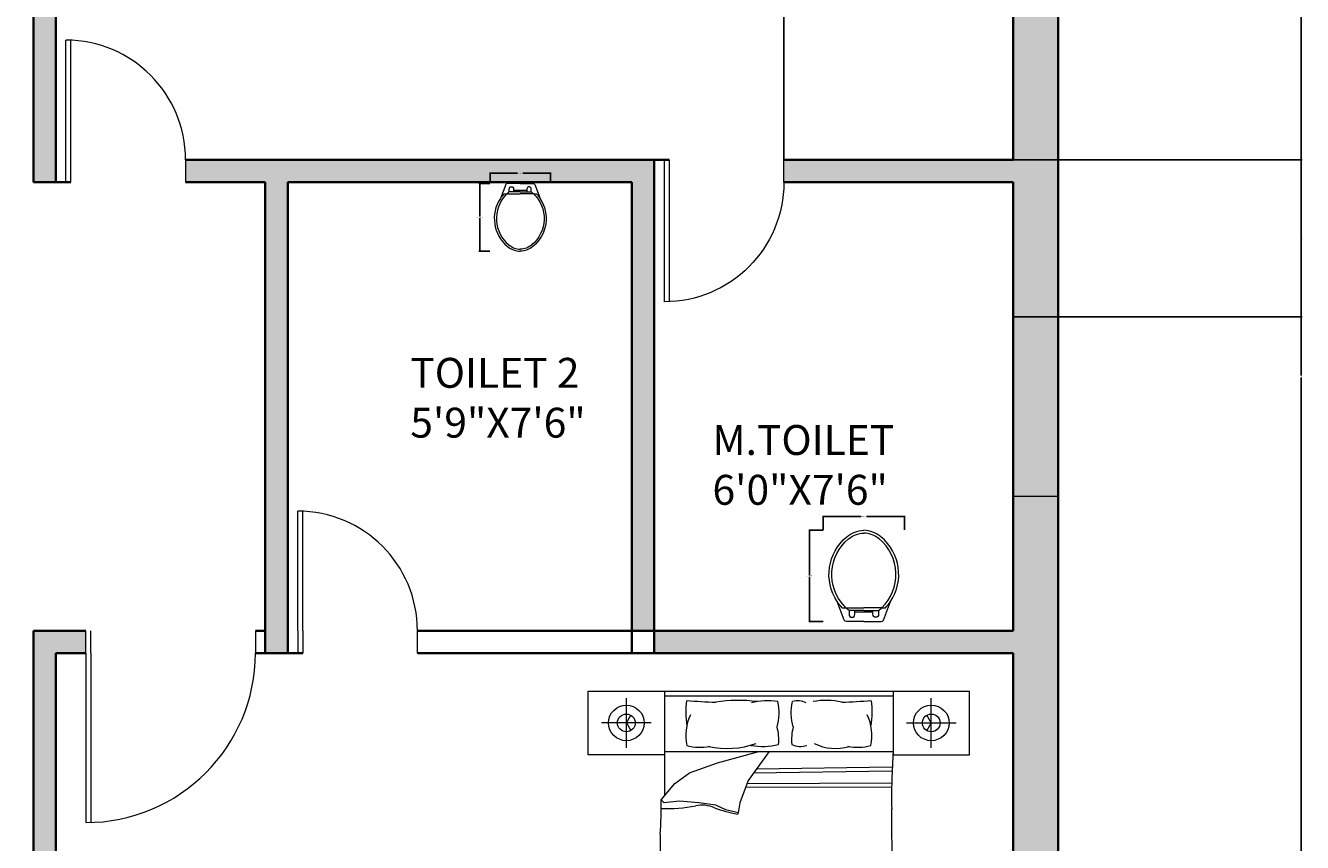
# Model space of a CAD drawing. Units: inches. Extents: x -26 to 13070, y -956 to 6917.
# Tile 4 of 13: x 341 to 597, y -760 to -596. Entities that reach past the tile are written whole.
import ezdxf

# ---------------------------------------------------------------- set-up
doc = ezdxf.new("R2010")
doc.units = ezdxf.units.IN
doc.header["$MEASUREMENT"] = 0
for name, color, linetype, lineweight in [('A-ANNO-DIMS', 2, 'Continuous', 18), ('A-AREA-IDEN', 7, 'Continuous', 18), ('A-DOOR', 3, 'Continuous', 18), ('A-FLOR-FIXT', 9, 'Continuous', 18), ('A-FURN', 8, 'Continuous', 13), ('A-GLAZ', 4, 'Continuous', 18), ('A-GLAZ-PATT', 8, 'Continuous', 13), ('A-WALL', 7, 'Continuous', 35), ('A-WALL-PATT', 252, 'Continuous', 13)]:
    doc.layers.add(name, color=color, linetype=linetype, lineweight=lineweight)
doc.styles.get("Standard").update_dxf_attribs({"font": 'arial.ttf'})
doc.dimstyles.get("Standard").update_dxf_attribs({"dimtxt": 0.18, "dimasz": 0.18, "dimexe": 0.18, "dimexo": 0.0625, "dimgap": 0.09, "dimtad": 0, "dimtih": 1, "dimtoh": 1, "dimdec": 0, "dimzin": 0, "dimdsep": 46, "dimlunit": 3, "dimtxsty": 'Standard', "dimcen": 0.09, "dimadec": 0, "dimazin": 0, "dimtfac": 1, "dimtdec": 0, "dimtofl": 0, "dimtmove": 0, "dimatfit": 3, "dimfxl": 1, "dimtolj": 1, "dimtzin": 0, "dimarcsym": 0})

# ---------------------------------------------------------------- blocks, each defined once
blk = doc.blocks.new('BED-DOUBLE-NIGHTSTANDS')
for p, q in [((0, 65), (76.43, 65)), ((15.29, 65), (15.29, 44.02)), ((7.64, 53.64), (7.64, 63.62)), ((61.14, 64.02), (15.29, 64.02)), ((68.79, 53.64), (68.79, 63.62)), ((12.64, 58.63), (2.65, 58.63)), ((63.79, 58.63), (73.78, 58.63)), ((15.29, 52.92), (61.14, 52.92)), ((25.9, 50.65), (34.24, 52.92)), ((36.28, 52.92), (32.09, 47.09)), ((20.33, 48.64), (25.9, 50.65)), ((60.91, 48.96), (33.16, 48.57)), ((60.94, 49.74), (33.73, 49.36)), ((14.6, 43.22), (17.39, 46.47)), ((17.39, 46.47), (20.33, 48.64)), ((32.09, 47.09), (30.39, 42.6)), ((60.87, 46.55), (31.85, 46.44)), ((60.87, 45.77), (31.55, 45.65)), ((15.22, 42.6), (14.6, 43.22)), ((18.32, 42.91), (15.22, 42.6)), ((22.19, 42.6), (18.32, 42.91)), ((25.59, 42.14), (22.19, 42.6)), ((27.6, 41.21), (25.59, 42.14)), ((30.08, 40.59), (27.6, 41.21)), ((30.39, 42.6), (30.08, 40.59)), ((10.09, 27.53), (14.41, 27.53)), ((10.09, 0), (10.09, 27.53)), ((14.41, 26.65), (10.97, 26.65)), ((10.97, 26.65), (10.97, 0.89)), ((64.92, 26.65), (61.55, 26.65)), ((61.57, 27.53), (65.81, 27.53)), ((64.92, 0.89), (64.92, 26.65)), ((65.81, 27.53), (65.81, 0)), ((61.56, 21.81), (14.4, 21.81)), ((61.49, 22.77), (14.41, 22.77)), ((53.73, 14.3), (22.7, 14.3)), ((18.51, 8.63), (18.34, 9.5)), ((23.85, 8.63), (24.02, 9.5)), ((52.05, 8.63), (51.88, 9.5)), ((57.39, 8.63), (57.56, 9.5)), ((10.97, 0.89), (64.92, 0.89)), ((65.81, 0), (10.09, 0))]:
    blk.add_line(p, q)
for points in [[(15.29, 52.26), (0, 52.26), (0, 65)], [(61.14, 65), (61.14, 52.26), (76.43, 52.26), (76.43, 65)], [(7.64, 58.63), (8.53, 60.17)], [(68.79, 58.63), (67.89, 60.17)], [(7.64, 58.63), (8.53, 57.08)], [(68.79, 58.63), (67.89, 57.08)]]:
    blk.add_lwpolyline(points)
for points in [[(19.68, 63.09, 0.074897), (19.77, 58.1, -0.472817)], [(37.86, 57.82, 0.14099), (38.01, 62.91, 0.235245)], [(41.12, 57.82, -0.14099), (40.97, 62.91, -0.235245)], [(56.75, 63.09, -0.074897), (56.66, 58.1, 0.472817)], [(14.44, 36.22, 0.001242), (14.4, 21.72, -0.127202), (12.87, 14.5)], [(61.47, 23.37, 0.056112), (62.02, 19.16, 0.095341), (63.1, 15.11)]]:
    blk.add_lwpolyline(points, format="xyb")
for centre, radius in [((7.64, 58.63), 3.57), ((68.79, 58.63), 3.57), ((7.64, 58.63), 1.78), ((68.79, 58.63), 1.78), ((22.92, 5.86), 0.195), ((52.98, 5.86), 0.195), ((21.65, 3.81), 0.195), ((54.25, 3.81), 0.195)]:
    blk.add_circle(centre, radius)
for centre, radius, start, end in [((61.8, 790.45), 728.57, 266.68521, 267.14978), ((30.15, 35.44), 27.72, 82.2196, 99.497), ((36, 49.44), 13.62, 81.5249, 103.96), ((42.02, 59.28), 3.78, 63.3437, 106.1026), ((47.68, 49.72), 13.44, 76.3427, 101.1841), ((14.63, 790.45), 728.57, 272.85022, 273.31479), ((29.41, 56.1), 9.85, 155.1316, 191.7583), ((47.02, 56.1), 9.85, 348.2417, 24.8684), ((28.85, 55.27), 9.36, 354.0129, 15.8293), ((50.13, 55.27), 9.36, 164.1707, 185.9871), ((22.4, 63.99), 10.24, 255.1039, 281.0369), ((27.79, 71.27), 17.76, 258.0397, 289.2615), ((34.99, 67.39), 13.48, 259.8617, 283.6238), ((42.53, 57.96), 4.05, 245.0183, 288.5407), ((49.61, 63.23), 9.73, 243.8761, 286.1746), ((54.03, 63.99), 10.24, 258.9631, 284.8961), ((198.16, 43.58), 137.33, 176.1, 180.9282), ((-55.48, 41.32), 70.1, 355.8294, 1.553), ((15.91, 70.29), 28.85, 267.4519, 281.3392), ((22.8, 35.91), 6.22, 66.2616, 101.3392), ((35.39, 69.47), 29.64, 250.1194, 259.3383), ((239.96, 38.59), 179.14, 179.1145, 184.8735), ((29.91, 40.53), 0.184, 268.8623, 19.7536), ((13.58, 14.54), 0.705, 183.98, 297.3412), ((21.79, -65.25), 79.56, 89.3433, 95.6887), ((16.65, 11.7), 1.29, 84.4856, 181.0538), ((13.28, 8.92), 5.78, 33.6671, 63.2997), ((16.25, 10.75), 2.3, 355.2933, 76.921), ((21.03, 12.36), 2.95, 145.785, 184.7304), ((15.4, 13.74), 3.17, 328.8218, 9.1554), ((19.32, 13.46), 0.92, 120.0293, 142.325), ((17.85, 12.92), 2.44, 289.2822, 29.1751), ((17.48, 12.48), 2.2, 7.436, 29.9149), ((18.93, 13.64), 1.14, 311.5653, 23.8354), ((19.32, 13.46), 0.92, 44.4517, 63.558), ((24.5, 12.92), 2.44, 150.8249, 250.7178), ((23.42, 13.64), 1.14, 156.1646, 228.4347), ((23.03, 13.46), 0.92, 113.229, 135.5483), ((24.87, 12.48), 2.2, 150.0851, 172.564), ((23.03, 13.46), 0.92, 37.675, 66.7144), ((21.32, 12.36), 2.95, 355.2696, 34.215), ((26.95, 13.74), 3.17, 169.7133, 211.1782), ((26.1, 10.75), 2.3, 103.079, 184.7067), ((29.07, 8.92), 5.78, 111.4941, 146.3329), ((25.7, 11.7), 1.29, 358.9462, 95.5144), ((50.19, 11.7), 1.29, 84.4856, 181.0538), ((46.82, 8.92), 5.78, 33.6671, 68.5059), ((49.8, 10.75), 2.3, 355.2933, 76.921), ((54.57, 12.36), 2.95, 145.785, 184.7304), ((48.94, 13.74), 3.17, 328.8218, 10.2867), ((52.87, 13.46), 0.92, 113.2856, 142.325), ((51.4, 12.92), 2.44, 289.2822, 29.1751), ((51.03, 12.48), 2.2, 7.436, 29.9149), ((52.87, 13.46), 0.92, 44.4517, 66.7144), ((52.48, 13.64), 1.14, 311.5653, 23.8354), ((56.07, -60.03), 74.37, 85.2402, 91.8035), ((58.04, 12.92), 2.44, 150.8249, 250.7178), ((56.96, 13.64), 1.14, 156.1646, 228.4347), ((56.57, 13.46), 0.92, 106.6343, 135.5483), ((58.41, 12.48), 2.2, 150.0851, 172.564), ((56.57, 13.46), 0.92, 37.675, 72.5814), ((54.87, 12.36), 2.95, 355.2696, 34.215), ((60.5, 13.74), 3.17, 169.249, 211.1782), ((59.64, 10.75), 2.3, 103.079, 184.7067), ((62.62, 8.92), 5.78, 113.6453, 146.3329), ((59.25, 11.7), 1.29, 358.9462, 95.5144), ((62.52, 14.72), 0.697, 246.5219, 33.8264), ((17.18, 11.52), 1.83, 174.9449, 262.8857), ((17.9, 12.21), 1.77, 201.5819, 291.4221), ((16.86, 11.92), 2.22, 272.3591, 324.0401), ((14.45, 10.81), 4.1, 326.2883, 356.5076), ((17.56, 10.28), 1.9, 299.9085, 73.1337), ((21.03, 12.36), 2.95, 212.7011, 216.3445), ((18.76, 11.08), 0.474, 257.3041, 15.1471), ((20.73, 11.61), 1.57, 131.5653, 195.1471), ((21.4, 10.36), 0.147, 102.7051, 280.4384), ((21.38, 10.45), 0.24, 280.4384, 100.4136), ((21.62, 11.61), 1.57, 344.8529, 48.4347), ((24.79, 10.28), 1.9, 106.8663, 240.0915), ((23.59, 11.08), 0.474, 164.8529, 282.6959), ((21.32, 12.36), 2.95, 323.6555, 327.2989), ((25.49, 11.92), 2.22, 215.9599, 267.6409), ((24.46, 12.21), 1.77, 248.5779, 338.4181), ((27.9, 10.81), 4.1, 183.4924, 213.7117), ((25.17, 11.52), 1.83, 277.1143, 5.0551), ((50.72, 11.52), 1.83, 174.9449, 262.8857), ((51.44, 12.21), 1.77, 201.5819, 291.4221), ((50.4, 11.92), 2.22, 272.3591, 324.0401), ((47.99, 10.81), 4.1, 326.2883, 356.5076), ((51.1, 10.28), 1.9, 299.9085, 73.1337), ((54.57, 12.36), 2.95, 212.7011, 216.3445), ((52.3, 11.08), 0.474, 257.3041, 15.1471), ((54.28, 11.61), 1.57, 131.5653, 195.1471), ((54.52, 10.45), 0.24, 79.5864, 259.5616), ((54.5, 10.36), 0.147, 259.5616, 77.2949), ((55.16, 11.61), 1.57, 344.8529, 48.4347), ((58.34, 10.28), 1.9, 106.8663, 240.0915), ((57.13, 11.08), 0.474, 164.8529, 282.6959), ((54.87, 12.36), 2.95, 323.6555, 327.2989), ((59.04, 11.92), 2.22, 215.9599, 267.6409), ((58, 12.21), 1.77, 248.5779, 338.4181), ((61.45, 10.81), 4.1, 183.4924, 213.7117), ((58.72, 11.52), 1.83, 277.1143, 5.0551), ((15.79, 6.99), 0.827, 92.9516, 193.728), ((14.09, 8.25), 1.7, 301.3827, 345.2969), ((16.76, 8.57), 1.15, 80.264, 250.8688), ((16.52, 7.33), 0.703, 63.9755, 143.2681), ((14.48, 11.1), 3.61, 301.2614, 341.7045), ((16.48, 8.92), 1.43, 265.969, 344.3045), ((18.02, 7.01), 1.53, 96.1662, 141.5825), ((19.47, 7.55), 0.15, 345.2356, 144.9248), ((20.55, 8.08), 0.401, 101.3256, 154.4621), ((19.97, 9.45), 1.21, 280.2588, 300.656), ((20.25, 10.41), 2.16, 268.3264, 277.1302), ((26.69, 6.51), 6.33, 163.5842, 183.8277), ((19.71, 9.44), 1.23, 308.2101, 316.3071), ((20.47, 8.64), 0.367, 278.3432, 4.2869), ((20.26, 8.96), 0.641, 300.656, 332.6341), ((20.74, 8.53), 0.156, 55.7657, 157.4417), ((26.69, 6.51), 6.33, 153.0032, 159.8941), ((20.99, 8.68), 0.156, 84.3784, 186.0543), ((20.84, 9.3), 0.641, 269.1859, 301.164), ((21.03, 8.97), 0.367, 237.5332, 323.4768), ((20.67, 10.02), 1.23, 285.5129, 293.6099), ((20.55, 9.79), 1.21, 301.164, 321.5612), ((21.48, 8.64), 0.401, 87.3579, 140.4944), ((19.56, 10), 2.16, 324.6898, 333.4936), ((27.87, 11.1), 3.61, 198.2955, 238.7386), ((24.33, 7.01), 1.53, 38.4175, 83.8338), ((25.87, 8.92), 1.43, 195.6955, 274.031), ((25.59, 8.57), 1.15, 289.1312, 99.736), ((25.83, 7.33), 0.703, 36.7319, 116.0245), ((26.57, 6.99), 0.827, 346.272, 87.0484), ((28.26, 8.25), 1.7, 194.7031, 238.6173), ((38.81, -0.46), 9.98, 94.4623, 172.255), ((38.85, 8.75), 1.11, 137.7873, 219.1145), ((37.6, 8.78), 0.834, 298.5391, 58.3627), ((38.83, 9.26), 0.827, 63.0274, 163.8037), ((37.99, 11.2), 1.7, 271.4585, 315.3727), ((38.68, 8.05), 1.58, 45.5411, 114.3101), ((40.12, 16.15), 6.98, 252.593, 267.2582), ((38.85, 9.46), 0.816, 177.7585, 283.852), ((40.42, 10.31), 2.52, 198.9159, 238.011), ((39.76, 8.05), 1.58, 65.6899, 134.4589), ((38.32, 16.15), 6.98, 272.7418, 287.407), ((39.02, 8.77), 0.108, 283.852, 219.9245), ((39.15, 8.27), 0.124, 238.011, 71.5592), ((39.17, 8.33), 0.0602, 71.5592, 188.0167), ((39.29, 8.27), 0.124, 108.4408, 301.989), ((39.62, 9.26), 0.827, 16.1963, 116.9726), ((40.45, 11.2), 1.7, 224.6273, 268.5415), ((39.27, 8.33), 0.0602, 351.9833, 108.4408), ((39.42, 8.81), 0.0651, 320.1909, 256.0209), ((38.02, 10.31), 2.52, 301.989, 341.0841), ((39.6, 9.46), 0.816, 256.148, 2.2415), ((40.85, 8.78), 0.834, 121.6373, 241.4609), ((39.59, 8.75), 1.11, 320.8855, 42.2127), ((39.31, 1.85), 7.72, 352.8636, 81.8197), ((49.33, 6.99), 0.827, 92.9516, 193.728), ((47.64, 8.25), 1.7, 301.3827, 345.2969), ((50.3, 8.57), 1.15, 80.264, 250.8688), ((50.06, 7.33), 0.703, 63.9755, 143.2681), ((48.03, 11.1), 3.61, 301.2614, 341.7045), ((50.03, 8.92), 1.43, 265.969, 344.3045), ((51.57, 7.01), 1.53, 96.1662, 141.5825), ((55.35, 9.79), 1.21, 218.4388, 238.836), ((54.42, 8.64), 0.401, 39.5056, 92.6421), ((56.33, 10), 2.16, 206.5064, 215.3102), ((54.87, 8.97), 0.367, 216.5232, 302.4668), ((55.05, 9.3), 0.641, 238.836, 270.8141), ((55.22, 10.02), 1.23, 246.3901, 254.4871), ((49.2, 6.51), 6.33, 20.1059, 26.9968), ((54.91, 8.68), 0.156, 353.9457, 95.6216), ((55.15, 8.53), 0.156, 22.5583, 124.2343), ((55.43, 8.64), 0.367, 175.7131, 261.6568), ((55.63, 8.96), 0.641, 207.3659, 239.344), ((49.2, 6.51), 6.33, 356.1723, 16.4158), ((56.18, 9.44), 1.23, 223.6929, 231.7899), ((55.92, 9.45), 1.21, 239.344, 259.7412), ((55.64, 10.41), 2.16, 262.8698, 271.6736), ((55.34, 8.08), 0.401, 25.5379, 78.6744), ((56.42, 7.55), 0.15, 35.0752, 194.7644), ((61.41, 11.1), 3.61, 198.2955, 238.7386), ((59.41, 8.92), 1.43, 195.6955, 274.031), ((57.87, 7.01), 1.53, 38.4175, 83.8338), ((59.14, 8.57), 1.15, 289.1312, 99.736), ((59.37, 7.33), 0.703, 36.7319, 116.0245), ((61.8, 8.25), 1.7, 194.7031, 238.6173), ((60.11, 6.99), 0.827, 346.272, 87.0484), ((3.54, -0.46), 9.98, 7.745, 41.8856), ((20.62, -1.45), 9.98, 124.3865, 158.5908), ((16.06, 6.55), 1.11, 167.7115, 249.0387), ((16.26, 5.87), 1.58, 75.4653, 144.2343), ((13.47, 13.61), 6.98, 282.5173, 297.1824), ((14.96, 5.96), 0.834, 328.4633, 88.2869), ((16.64, 8.69), 2.52, 228.8402, 267.9352), ((15.7, 7.17), 0.816, 207.6827, 313.7762), ((16.19, 6.66), 0.108, 313.7762, 249.7183), ((16.54, 6.35), 0.0602, 101.4834, 217.9409), ((16.56, 6.29), 0.124, 267.9352, 101.4834), ((19.42, 7.32), 0.325, 101.5637, 142.6358), ((19.15, 7.02), 0.195, 273.2768, 86.7232), ((19.41, 6.66), 0.321, 217.7621, 259.0403), ((19.37, 7.21), 0.186, 91.1081, 181.8675), ((19.76, 7.09), 0.591, 203.4276, 227.6104), ((19.57, 6.83), 0.402, 80.3487, 133.6538), ((19.5, 7.16), 0.318, 229.7889, 317.6792), ((19.16, 7.58), 0.468, 288.7263, 352.5032), ((19.14, 6.49), 0.452, 355.053, 68.3618), ((19.5, 6.41), 0.637, 83.0852, 105.7171), ((19.44, 6.46), 0.149, 232.4737, 355.053), ((15.08, 1.13), 7.26, 43.1541, 52.0459), ((19.61, 7.06), 0.168, 317.6792, 80.3487), ((20.1, 5.51), 0.401, 101.3256, 154.4621), ((19.52, 6.87), 1.21, 280.2588, 300.656), ((19.8, 7.84), 2.16, 268.3264, 277.1302), ((19.26, 6.87), 1.23, 308.2101, 316.3071), ((20.01, 6.06), 0.367, 278.3432, 4.2869), ((19.81, 6.39), 0.641, 300.656, 332.6341), ((20.29, 5.96), 0.156, 55.7657, 157.4417), ((23.54, 6.35), 3.17, 184.756, 209.2041), ((28.11, 13.11), 10.44, 222.2412, 232.1744), ((23.87, 2.14), 3.81, 120.544, 139.818), ((21.43, 6.15), 0.887, 304.5369, 16.3699), ((21.9, 5.96), 0.539, 272.8499, 356.1226), ((21.52, 5.75), 0.522, 321.7607, 7.9252), ((21.63, 5), 0.522, 8.7227, 54.8872), ((21.66, 4.58), 0.887, 0.278, 72.111), ((22.66, 5.9), 0.628, 127.3105, 187.9252), ((22.06, 4.9), 0.539, 20.5253, 88.5375), ((21.8, 5.98), 0.645, 355.0106, 41.658), ((22.51, 5.5), 0.193, 148.0499, 225.6268), ((23.87, 2.14), 3.81, 113.0501, 113.8477), ((22.87, 5.28), 0.614, 104.7558, 148.0499), ((22.52, 5.72), 0.384, 247.4086, 351.4386), ((22.71, 6.14), 0.265, 126.1046, 271.4281), ((22.68, 6.21), 0.191, 353.7526, 131.7054), ((22.63, 5.7), 0.129, 262.906, 7.132), ((22.5, 5.98), 0.268, 0.0645, 61.1507), ((22.56, 6.21), 0.306, 311.8413, 355.7877), ((23.19, 5.5), 0.321, 151.2196, 259.0403), ((23.19, 6.17), 0.325, 101.5637, 176.365), ((23.15, 6.05), 0.186, 91.1081, 181.8675), ((23.53, 5.93), 0.591, 203.4276, 227.6104), ((23.35, 5.67), 0.402, 80.3487, 133.6538), ((23.27, 6.01), 0.318, 229.7889, 317.6792), ((22.93, 6.42), 0.468, 288.7263, 352.5032), ((22.91, 5.33), 0.452, 355.053, 68.3618), ((23.27, 5.26), 0.637, 83.0852, 105.7171), ((23.25, 6.4), 0.15, 345.2356, 144.9248), ((23.22, 5.31), 0.149, 232.4737, 355.053), ((23.38, 5.91), 0.168, 317.6792, 80.3487), ((23.87, 2.14), 3.81, 87.1071, 94.7585), ((25.8, 6.29), 0.124, 78.5166, 272.0648), ((26.09, 5.87), 1.58, 35.7657, 104.5347), ((28.88, 13.61), 6.98, 242.8176, 257.4827), ((25.71, 8.69), 2.52, 272.0648, 311.1598), ((25.81, 6.35), 0.0602, 322.0591, 78.5166), ((26.65, 7.17), 0.816, 226.2238, 332.3173), ((26.17, 6.7), 0.0651, 290.2667, 226.2271), ((27.4, 5.96), 0.834, 91.7131, 211.5367), ((26.29, 6.55), 1.11, 290.9613, 12.2885), ((21.73, -1.45), 9.98, 21.4092, 55.6135), ((54.16, -1.45), 9.98, 124.3865, 158.5908), ((49.61, 6.55), 1.11, 167.7115, 249.0387), ((49.81, 5.87), 1.58, 75.4653, 144.2343), ((47.01, 13.61), 6.98, 282.5173, 297.1824), ((49.25, 7.17), 0.816, 207.6827, 313.7762), ((50.19, 8.69), 2.52, 228.8402, 267.9352), ((48.5, 5.96), 0.834, 328.4633, 88.2869), ((49.74, 6.66), 0.108, 313.7762, 249.7183), ((50.09, 6.35), 0.0602, 101.4834, 217.9409), ((50.1, 6.29), 0.124, 267.9352, 101.4834), ((52.03, 2.14), 3.81, 85.2415, 92.8929), ((52.51, 5.91), 0.168, 99.6513, 222.3208), ((52.62, 6.01), 0.318, 222.3208, 310.2111), ((52.55, 5.67), 0.402, 46.3462, 99.6513), ((52.65, 6.4), 0.15, 35.0752, 194.7644), ((52.97, 6.42), 0.468, 187.4968, 251.2737), ((52.98, 5.33), 0.452, 111.6382, 184.947), ((52.68, 5.31), 0.149, 184.947, 307.5263), ((52.63, 5.26), 0.637, 74.2829, 96.9148), ((52.75, 6.05), 0.186, 358.1325, 88.8919), ((52.36, 5.93), 0.591, 312.3896, 336.5724), ((52.71, 6.17), 0.325, 3.635, 78.4363), ((52.71, 5.5), 0.321, 280.9597, 28.7804), ((53.37, 5.72), 0.384, 188.5614, 292.5914), ((53.22, 6.21), 0.191, 48.2946, 186.2474), ((53.34, 6.21), 0.306, 184.2123, 228.1587), ((53.4, 5.98), 0.268, 118.8493, 179.9355), ((53.26, 5.7), 0.129, 172.868, 277.094), ((53.19, 6.14), 0.265, 268.5719, 53.8954), ((53.03, 5.28), 0.614, 31.9501, 75.2442), ((53.84, 4.9), 0.539, 91.4625, 159.4747), ((54.23, 4.58), 0.887, 107.889, 179.722), ((54.1, 5.98), 0.645, 138.342, 184.9894), ((53.99, 5.96), 0.539, 183.8774, 267.1501), ((52.03, 2.14), 3.81, 66.1523, 66.9499), ((53.38, 5.5), 0.193, 314.3732, 31.9501), ((54.47, 6.15), 0.887, 163.6301, 235.4631), ((53.23, 5.9), 0.628, 352.0748, 52.6895), ((54.26, 5), 0.522, 125.1128, 171.2773), ((54.37, 5.75), 0.522, 172.0748, 218.2393), ((52.03, 2.14), 3.81, 40.182, 59.456), ((47.79, 13.11), 10.44, 307.8256, 317.7588), ((52.36, 6.35), 3.17, 330.7959, 355.244), ((60.81, 1.13), 7.26, 127.9541, 136.8459), ((55.61, 5.96), 0.156, 22.5583, 124.2343), ((55.88, 6.06), 0.367, 175.7131, 261.6568), ((56.09, 6.39), 0.641, 207.3659, 239.344), ((56.64, 6.87), 1.23, 223.6929, 231.7899), ((56.38, 6.87), 1.21, 239.344, 259.7412), ((56.1, 7.84), 2.16, 262.8698, 271.6736), ((55.8, 5.51), 0.401, 25.5379, 78.6744), ((56.28, 7.06), 0.168, 99.6513, 222.3208), ((56.4, 7.16), 0.318, 222.3208, 310.2111), ((56.32, 6.83), 0.402, 46.3462, 99.6513), ((56.74, 7.58), 0.468, 187.4968, 251.2737), ((56.76, 6.49), 0.452, 111.6382, 184.947), ((56.45, 6.46), 0.149, 184.947, 307.5263), ((56.4, 6.41), 0.637, 74.2829, 96.9148), ((56.52, 7.21), 0.186, 358.1325, 88.8919), ((56.14, 7.09), 0.591, 312.3896, 336.5724), ((56.48, 7.32), 0.325, 37.3642, 78.4363), ((56.48, 6.66), 0.321, 280.9597, 322.2379), ((56.75, 7.02), 0.195, 93.2768, 266.7232), ((59.34, 6.29), 0.124, 78.5166, 272.0648), ((59.63, 5.87), 1.58, 35.7657, 104.5347), ((62.43, 13.61), 6.98, 242.8176, 257.4827), ((59.25, 8.69), 2.52, 272.0648, 311.1598), ((59.35, 6.35), 0.0602, 322.0591, 78.5166), ((60.19, 7.17), 0.816, 226.2238, 332.3173), ((59.71, 6.7), 0.0651, 290.2667, 226.2271), ((60.94, 5.96), 0.834, 91.7131, 211.5367), ((59.83, 6.55), 1.11, 290.9613, 12.2885), ((55.28, -1.45), 9.98, 21.4092, 55.6135), ((72.35, -0.46), 9.98, 138.1144, 172.255), ((20.23, 4.81), 0.217, 146.8636, 236.9021), ((23.3, 9.6), 5.69, 235.1882, 238.8844), ((20.6, 5.12), 0.588, 199.4799, 267.6828), ((20.54, 4.9), 0.507, 212.8155, 277.3992), ((20.24, 4.56), 0.588, 266.9701, 338.2913), ((17.14, 8.76), 5.69, 302.6784, 306.3746), ((20.39, 4.1), 0.217, 214.3538, 304.3923), ((20.47, 4.92), 0.225, 238.8844, 314.2646), ((20.42, 4.42), 0.507, 280.3057, 17.1958), ((20.38, 4.36), 0.225, 306.3746, 21.7548), ((20.75, 4.51), 0.17, 19.3605, 201.7548), ((20.75, 4.64), 0.17, 311.8703, 134.2646), ((23.94, 3.09), 3.39, 153.7819, 158.2913), ((21.24, 5.41), 0.887, 247.2305, 319.0635), ((20.95, 5.11), 0.522, 264.4544, 310.6188), ((23.54, 6.35), 3.17, 214.0033, 222.4917), ((21.33, 4.9), 0.539, 218.3208, 298.8162), ((21.24, 3.45), 0.193, 148.0499, 225.6268), ((21.6, 3.23), 0.614, 104.7558, 148.0499), ((21.25, 3.66), 0.384, 247.4086, 351.4386), ((21.43, 4.08), 0.265, 126.1046, 271.4281), ((21.4, 4.16), 0.191, 353.7526, 131.7054), ((21.7, 4.23), 0.628, 70.0041, 130.6188), ((21.36, 3.65), 0.129, 262.906, 7.132), ((21.22, 3.93), 0.268, 0.0645, 61.1507), ((21.29, 4.16), 0.306, 311.8413, 355.7877), ((21.29, 5), 0.645, 297.7043, 344.3516), ((21.92, 4.11), 0.325, 101.5637, 176.365), ((21.91, 3.45), 0.321, 151.2196, 259.0403), ((21.87, 4), 0.186, 91.1081, 181.8675), ((22.26, 3.88), 0.591, 203.4276, 227.6104), ((22.07, 3.62), 0.402, 80.3487, 133.6538), ((22, 3.96), 0.318, 229.7889, 317.6792), ((21.66, 4.37), 0.468, 288.7263, 352.5032), ((21.64, 3.28), 0.452, 355.053, 68.3618), ((22, 3.21), 0.637, 83.0852, 105.7171), ((21.97, 4.35), 0.15, 345.2356, 144.9248), ((21.94, 3.26), 0.149, 232.4737, 355.053), ((22.11, 3.85), 0.168, 317.6792, 80.3487), ((22.77, 5.17), 0.628, 188.7227, 249.3375), ((21.96, 4.86), 0.645, 334.9899, 21.6373), ((33.8, -1.8), 4.86, 91.272, 146.5383), ((35.55, -2.7), 6.06, 107.8504, 143.6964), ((38.74, -4.41), 9.02, 124.0123, 144.053), ((38.04, -5.81), 9.98, 94.4623, 117.4146), ((38.09, 3.4), 1.11, 137.7873, 219.1145), ((36.83, 3.44), 0.834, 298.5391, 58.3627), ((38.06, 3.91), 0.827, 63.0274, 163.8037), ((37.22, 5.85), 1.7, 271.4585, 315.3727), ((37.92, 2.71), 1.58, 45.5411, 114.3101), ((39.66, 4.96), 2.52, 198.9159, 238.011), ((39.36, 10.81), 6.98, 252.593, 267.2582), ((38.08, 4.11), 0.816, 177.7585, 283.852), ((38.25, 3.43), 0.108, 283.852, 219.9245), ((38.38, 2.93), 0.124, 238.011, 71.5592), ((38.4, 2.99), 0.0602, 71.5592, 188.0167), ((40.53, 2.71), 1.58, 65.6899, 134.4589), ((39.09, 10.81), 6.98, 272.7418, 287.407), ((40.06, 2.93), 0.124, 108.4408, 301.989), ((40.38, 3.91), 0.827, 16.1963, 116.9726), ((41.22, 5.85), 1.7, 224.6273, 268.5415), ((40.04, 2.99), 0.0602, 351.9833, 108.4408), ((40.18, 3.47), 0.0651, 320.1909, 256.0209), ((38.79, 4.96), 2.52, 301.989, 341.0841), ((40.36, 4.11), 0.816, 256.148, 2.2415), ((41.61, 3.44), 0.834, 121.6373, 241.4609), ((40.36, 3.4), 1.11, 320.8855, 42.2127), ((40.4, -5.81), 9.98, 62.5854, 85.5377), ((40.31, 2.55), 4.47, 338.117, 6.6195), ((44.41, 1.31), 1.79, 346.3898, 79.0739), ((43.06, 1.55), 2.27, 342.8609, 41.9049), ((53.93, 4.86), 0.645, 158.3627, 205.0101), ((53.13, 5.17), 0.628, 290.6625, 351.2773), ((53.78, 3.85), 0.168, 99.6513, 222.3208), ((53.9, 3.96), 0.318, 222.3208, 310.2111), ((53.82, 3.62), 0.402, 46.3462, 99.6513), ((53.92, 4.35), 0.15, 35.0752, 194.7644), ((54.24, 4.37), 0.468, 187.4968, 251.2737), ((54.26, 3.28), 0.452, 111.6382, 184.947), ((53.95, 3.26), 0.149, 184.947, 307.5263), ((53.9, 3.21), 0.637, 74.2829, 96.9148), ((54.2, 4.23), 0.628, 49.3812, 109.9959), ((54.65, 5.41), 0.887, 220.9365, 292.7695), ((54.6, 5), 0.645, 195.6484, 242.2957), ((54.02, 4), 0.186, 358.1325, 88.8919), ((53.64, 3.88), 0.591, 312.3896, 336.5724), ((53.98, 4.11), 0.325, 3.635, 78.4363), ((53.98, 3.45), 0.321, 280.9597, 28.7804), ((54.64, 3.66), 0.384, 188.5614, 292.5914), ((54.56, 4.9), 0.539, 241.1838, 321.6792), ((54.49, 4.16), 0.191, 48.2946, 186.2474), ((54.61, 4.16), 0.306, 184.2123, 228.1587), ((54.67, 3.93), 0.268, 118.8493, 179.9355), ((54.54, 3.65), 0.129, 172.868, 277.094), ((54.46, 4.08), 0.265, 268.5719, 53.8954), ((54.3, 3.23), 0.614, 31.9501, 75.2442), ((54.95, 5.11), 0.522, 229.3812, 275.5456), ((52.36, 6.35), 3.17, 317.5083, 325.9967), ((54.66, 3.45), 0.193, 314.3732, 31.9501), ((55.47, 4.42), 0.507, 162.8042, 259.6943), ((55.15, 4.64), 0.17, 45.7354, 228.1297), ((55.15, 4.51), 0.17, 338.2452, 160.6395), ((51.96, 3.09), 3.39, 21.7087, 26.2181), ((55.65, 4.56), 0.588, 201.7087, 273.0299), ((55.42, 4.92), 0.225, 225.7354, 301.1156), ((55.36, 4.9), 0.507, 262.6008, 327.1845), ((55.51, 4.36), 0.225, 158.2452, 233.6254), ((55.29, 5.12), 0.588, 272.3172, 340.5201), ((58.75, 8.76), 5.69, 233.6254, 237.3216), ((55.5, 4.1), 0.217, 235.6077, 325.6462), ((52.6, 9.6), 5.69, 301.1156, 304.8118), ((55.66, 4.81), 0.217, 303.0979, 33.1364), ((8.55, -1.8), 4.86, 33.4617, 60.1116), ((6.8, -2.7), 6.06, 36.3036, 46.4814), ((11.27, -0.67), 4.06, 22.5547, 48.9546), ((0.16, 1.51), 13.81, 357.4081, 3.6519), ((31.08, -0.67), 4.06, 131.0454, 157.4453), ((42.19, 1.51), 13.81, 176.3481, 182.5919), ((35.25, -4.36), 5.49, 73.5431, 107.0202), ((37.43, -7.19), 8.12, 94.3787, 95.6357), ((41.7, -12.75), 14.5, 109.7217, 109.9028), ((43.19, -4.36), 5.49, 72.9798, 106.4569), ((41.02, -7.19), 8.12, 84.3643, 85.6213), ((36.74, -12.75), 14.5, 70.0972, 70.2783), ((33.7, 1.51), 13.81, 357.4081, 3.6519), ((44.82, -0.67), 4.06, 22.5547, 48.9546), ((64.62, -0.67), 4.06, 131.0454, 157.4453), ((75.74, 1.51), 13.81, 176.3481, 182.5919), ((67.35, -1.8), 4.86, 119.8884, 146.5383), ((69.1, -2.7), 6.06, 133.5186, 143.6964)]:
    blk.add_arc(centre, radius, start, end)
blk = doc.blocks.new('WC-COMPACT')
for p, q in [((1.95, 11.55), (2.52, 11.55)), ((2.52, 11.55), (5.2, 11.55)), ((7.87, 11.55), (5.2, 11.55)), ((7.87, 11.55), (8.44, 11.55))]:
    blk.add_line(p, q)
for points in [[(5.2, 13.61), (2.6, 13.61, 0.31031), (2.28, 13.39), (1.21, 10.61, 0.209071)], [(2.99, 11.96), (2.99, 12.53, -1), (3.86, 12.53), (3.86, 12.23)], [(5.2, 13.61), (7.79, 13.61, -0.31031), (8.11, 13.39), (9.18, 10.61, -0.209071)], [(7.4, 11.96), (7.4, 12.53, 1), (6.54, 12.53), (6.54, 12.23)], [(1.21, 10.61, 0.383919), (2.64, 0.98, 0.163732), (5.2, 0, 0.359733)], [(2.25, 11.27, 0.431639), (2.9, 1.29, 0.162618), (5.2, 0.41, 0.470877)], [(1.95, 11.55, 0.040937), (1.21, 10.61, 0.163732)], [(2.52, 11.55, 0.014165), (2.25, 11.27, 0.162618)], [(2.99, 11.96, 0.022712), (2.52, 11.55, 0.162618)], [(5.2, 11.96), (2.99, 11.96, 0.022712)], [(5.2, 11.96), (7.4, 11.96, -0.476108)], [(7.87, 11.55, -0.448546), (7.5, 1.29, -0.162618), (5.2, 0.41, -0.470877)], [(9.18, 10.61, -0.383919), (7.75, 0.98, -0.163732), (5.2, 0, -0.359733)], [(7.4, 11.96, -0.022712), (7.87, 11.55, -0.162618)], [(8.44, 11.55, -0.040937), (9.18, 10.61, -0.163732)]]:
    blk.add_lwpolyline(points, format="xyb")
for points in [[(6.54, 12.23), (3.86, 12.23)], [(3.86, 12.23), (3.86, 11.96)], [(6.54, 12.23), (6.54, 11.96)]]:
    blk.add_lwpolyline(points)
blk = doc.blocks.new('WC-STANDARD')
for p, q in [((2.62, 2.77), (3.39, 2.77)), ((3.39, 2.77), (6.99, 2.77)), ((10.59, 2.77), (6.99, 2.77)), ((10.59, 2.77), (11.36, 2.77))]:
    blk.add_line(p, q)
for points in [[(1.63, 4.03, -0.383919), (3.55, 16.99, -0.163732), (6.99, 18.31, -0.359733)], [(12.35, 4.03, 0.383919), (10.43, 16.99, 0.163732), (6.99, 18.31, 0.359733)], [(3.02, 3.15, -0.431639), (3.9, 16.57, -0.162618), (6.99, 17.76, -0.470877)], [(10.59, 2.77, 0.448546), (10.08, 16.57, 0.162618), (6.99, 17.76, 0.470877)], [(2.62, 2.77, -0.040937), (1.63, 4.03, -0.163732)], [(6.99, 0), (3.49, 0, -0.31031), (3.07, 0.29), (1.63, 4.03, -0.209071)], [(3.39, 2.77, -0.014165), (3.02, 3.15, -0.162618)], [(4.02, 2.22, -0.022712), (3.39, 2.77, -0.162618)], [(6.99, 0), (10.49, 0, 0.31031), (10.92, 0.29), (12.35, 4.03, 0.209071)], [(9.96, 2.22, 0.022712), (10.59, 2.77, 0.162618)], [(11.36, 2.77, 0.040937), (12.35, 4.03, 0.163732)], [(6.99, 2.22), (4.02, 2.22, -0.022712)], [(4.02, 2.22), (4.02, 1.45, 1), (5.19, 1.45), (5.19, 1.85)], [(6.99, 2.22), (9.96, 2.22, 0.476108)], [(9.96, 2.22), (9.96, 1.45, -1), (8.79, 1.45), (8.79, 1.85)]]:
    blk.add_lwpolyline(points, format="xyb")
for points in [[(5.19, 1.85), (5.19, 2.22)], [(8.79, 1.85), (5.19, 1.85)], [(8.79, 1.85), (8.79, 2.22)]]:
    blk.add_lwpolyline(points)
blk = doc.blocks.new('DOOR-SWING-24')
for p, q in [((24, 1), (0, 1)), ((24, 0), (0, 0))]:
    blk.add_line(p, q)
blk.add_arc((24, 0), 24, 90, 180)
blk = doc.blocks.new('*D28')
at = {"layer": 'A-ANNO-DIMS', "color": 0, "lineweight": -2, "transparency": 16777216}
for p, q in [((433.65, -627.3), (431.49, -627.3)), ((431.67, -627.48), (431.67, -633.92)), ((431.67, -640.73), (431.67, -634.29)), ((433.65, -640.91), (431.49, -640.91))]:
    blk.add_line(p, q, dxfattribs=at)
at = {"layer": 'A-ANNO-DIMS', "color": 0, "transparency": 16777216}
for points in [[(431.64, -627.48), (431.7, -627.48), (431.67, -627.3)], [(431.64, -640.73), (431.7, -640.73), (431.67, -640.91)]]:
    blk.add_solid(points, dxfattribs=at)
at = {"layer": 'Defpoints', "color": 0, "transparency": 16777216}
for p in [(431.67, -627.3), (433.72, -627.3), (433.72, -640.91)]:
    blk.add_point(p, dxfattribs=at)
at = {"layer": 'A-ANNO-DIMS', "color": 0, "transparency": 16777216, "insert": (431.67, -634.11), "char_height": 0.18, "attachment_point": 5}
blk.add_mtext('\\A1;WC 14 TYP.', dxfattribs=at)
blk = doc.blocks.new('*D29')
at = {"layer": 'A-ANNO-DIMS', "color": 0, "lineweight": -2, "transparency": 16777216}
for p, q in [((433.72, -627.24), (433.72, -625.08)), ((433.9, -625.26), (439.24, -625.26)), ((445.63, -625.26), (440.28, -625.26)), ((445.81, -627.24), (445.81, -625.08))]:
    blk.add_line(p, q, dxfattribs=at)
at = {"layer": 'A-ANNO-DIMS', "color": 0, "transparency": 16777216}
for points in [[(433.9, -625.23), (433.9, -625.29), (433.72, -625.26)], [(445.63, -625.23), (445.63, -625.29), (445.81, -625.26)]]:
    blk.add_solid(points, dxfattribs=at)
at = {"layer": 'Defpoints', "color": 0, "transparency": 16777216}
for p in [(433.72, -627.3), (445.81, -625.26), (445.81, -627.3)]:
    blk.add_point(p, dxfattribs=at)
at = {"layer": 'A-ANNO-DIMS', "color": 0, "transparency": 16777216, "insert": (439.76, -625.26), "char_height": 0.18, "attachment_point": 5}
blk.add_mtext('\\A1;12 TYP.', dxfattribs=at)
blk = doc.blocks.new('*D30')
at = {"layer": 'A-ANNO-DIMS', "color": 0, "lineweight": -2, "transparency": 16777216}
for p, q in [((500.48, -696.9), (497.61, -696.9)), ((497.79, -697.08), (497.79, -705.87)), ((497.79, -715.03), (497.79, -706.23)), ((500.48, -715.21), (497.61, -715.21))]:
    blk.add_line(p, q, dxfattribs=at)
at = {"layer": 'A-ANNO-DIMS', "color": 0, "transparency": 16777216}
for points in [[(497.76, -697.08), (497.82, -697.08), (497.79, -696.9)], [(497.76, -715.03), (497.82, -715.03), (497.79, -715.21)]]:
    blk.add_solid(points, dxfattribs=at)
at = {"layer": 'Defpoints', "color": 0, "transparency": 16777216}
for p in [(497.79, -696.9), (500.54, -696.9), (500.54, -715.21)]:
    blk.add_point(p, dxfattribs=at)
at = {"layer": 'A-ANNO-DIMS', "color": 0, "transparency": 16777216, "insert": (497.79, -706.05), "char_height": 0.18, "attachment_point": 5}
blk.add_mtext('\\A1;WC 18 TYP.', dxfattribs=at)
blk = doc.blocks.new('*D31')
at = {"layer": 'A-ANNO-DIMS', "color": 0, "lineweight": -2, "transparency": 16777216}
for p, q in [((500.54, -696.83), (500.54, -693.97)), ((500.72, -694.15), (508.15, -694.15)), ((516.63, -694.15), (509.19, -694.15)), ((516.81, -696.83), (516.81, -693.97))]:
    blk.add_line(p, q, dxfattribs=at)
at = {"layer": 'A-ANNO-DIMS', "color": 0, "transparency": 16777216}
for points in [[(500.72, -694.12), (500.72, -694.18), (500.54, -694.15)], [(516.63, -694.12), (516.63, -694.18), (516.81, -694.15)]]:
    blk.add_solid(points, dxfattribs=at)
at = {"layer": 'Defpoints', "color": 0, "transparency": 16777216}
for p in [(516.81, -694.15), (500.54, -696.9), (516.81, -696.9)]:
    blk.add_point(p, dxfattribs=at)
at = {"layer": 'A-ANNO-DIMS', "color": 0, "transparency": 16777216, "insert": (508.67, -694.15), "char_height": 0.18, "attachment_point": 5}
blk.add_mtext('\\A1;16 TYP.', dxfattribs=at)
blk = doc.blocks.new('*D46')
at = {"layer": 'A-ANNO-DIMS', "color": 0, "lineweight": -2, "transparency": 16777216}
for p, q in [((538.7, -457.54), (596.57, -457.54)), ((596.39, -457.72), (596.39, -665.86)), ((596.39, -874.36), (596.39, -666.22)), ((547.7, -874.54), (596.57, -874.54))]:
    blk.add_line(p, q, dxfattribs=at)
at = {"layer": 'A-ANNO-DIMS', "color": 0, "transparency": 16777216}
for points in [[(596.36, -457.72), (596.42, -457.72), (596.39, -457.54)], [(596.36, -874.36), (596.42, -874.36), (596.39, -874.54)]]:
    blk.add_solid(points, dxfattribs=at)
at = {"layer": 'Defpoints', "color": 0, "transparency": 16777216}
for p in [(538.64, -457.54), (596.39, -457.54), (547.64, -874.54)]:
    blk.add_point(p, dxfattribs=at)
at = {"layer": 'A-ANNO-DIMS', "color": 0, "transparency": 16777216, "insert": (596.39, -666.04), "char_height": 0.18, "attachment_point": 5}
blk.add_mtext('\\A1;417', dxfattribs=at)
blk = doc.blocks.new('*D53')
at = {"layer": 'A-ANNO-DIMS', "color": 0, "lineweight": -2, "transparency": 16777216}
for p, q in [((492.64, -622.48), (492.64, 116.39)), ((492.82, 116.21), (515.42, 116.21)), ((538.46, 116.21), (515.86, 116.21)), ((538.64, -622.48), (538.64, 116.39))]:
    blk.add_line(p, q, dxfattribs=at)
at = {"layer": 'A-ANNO-DIMS', "color": 0, "transparency": 16777216}
for points in [[(492.82, 116.24), (492.82, 116.18), (492.64, 116.21)], [(538.46, 116.24), (538.46, 116.18), (538.64, 116.21)]]:
    blk.add_solid(points, dxfattribs=at)
at = {"layer": 'Defpoints', "color": 0, "transparency": 16777216}
for p in [(538.64, 116.21), (492.64, -622.54), (538.64, -622.54)]:
    blk.add_point(p, dxfattribs=at)
at = {"layer": 'A-ANNO-DIMS', "color": 0, "transparency": 16777216, "insert": (515.64, 116.21), "char_height": 0.18, "attachment_point": 5}
blk.add_mtext('\\A1;46', dxfattribs=at)
blk = doc.blocks.new('*D54')
at = {"layer": 'A-ANNO-DIMS', "color": 0, "lineweight": -2, "transparency": 16777216}
for p, q in [((538.7, -622.54), (596.57, -622.54)), ((596.39, -622.72), (596.39, -638.11)), ((596.39, -653.86), (596.39, -638.47)), ((538.7, -654.04), (596.57, -654.04))]:
    blk.add_line(p, q, dxfattribs=at)
at = {"layer": 'A-ANNO-DIMS', "color": 0, "transparency": 16777216}
for points in [[(596.36, -622.72), (596.42, -622.72), (596.39, -622.54)], [(596.36, -653.86), (596.42, -653.86), (596.39, -654.04)]]:
    blk.add_solid(points, dxfattribs=at)
at = {"layer": 'Defpoints', "color": 0, "transparency": 16777216}
for p in [(538.64, -622.54), (596.39, -622.54), (538.64, -654.04)]:
    blk.add_point(p, dxfattribs=at)
at = {"layer": 'A-ANNO-DIMS', "color": 0, "transparency": 16777216, "insert": (596.39, -638.29), "char_height": 0.18, "attachment_point": 5}
blk.add_mtext('\\A1;31.5', dxfattribs=at)

msp = doc.modelspace()

# ---------------------------------------------------------------- hatches: boundary and pattern name
at = {"layer": 'A-GLAZ-PATT'}
h = msp.add_hatch(dxfattribs=at)
h.set_pattern_fill('GOST_WOOD', color=256)
h.set_pattern_definition([(90, (0, 0), (6, -4e-16), [10, -2]), (90, (2, -2), (6, -4e-16), [6, -1.5, 3, -1.5]), (90, (4, -5), (6, -4e-16), [10, -2])])
h.paths.add_polyline_path([(547.641, -159.042), (538.641, -159.042), (538.641, -195.042), (547.641, -195.042)])
h.paths.add_polyline_path([(547.641, -234.042), (538.641, -234.042), (538.641, -270.042), (547.641, -270.042)])
h.paths.add_polyline_path([(547.641, -654.042), (538.641, -654.042), (538.641, -690.042), (547.641, -690.042)])
at = {"layer": 'A-WALL-PATT'}
h = msp.add_hatch(color=256, dxfattribs=at)
h.dxf.hatch_style = 1
h.paths.add_polyline_path([(223.641, 10.458), (214.641, 10.458), (22.641, 10.458), (22.641, -171.042), (31.641, -171.042), (31.641, -135.042), (205.641, -135.042), (205.641, -241.042), (210.141, -241.042), (210.141, -130.542), (94.641, -130.542), (94.641, -76.542), (85.641, -76.542), (85.641, -126.042), (27.141, -126.042), (27.141, 5.958), (85.641, 5.958), (85.641, -52.542), (94.641, -52.542), (94.641, 1.458), (214.641, 1.458), (214.641, -16.542), (223.641, -16.542), (229.641, -16.542), (229.641, -7.542), (223.641, -7.542)])
h.paths.add_polyline_path([(367.048, 10.458), (346.641, 10.458), (337.641, 10.458), (337.641, -7.542), (331.641, -7.542), (331.641, -16.542), (337.641, -16.542), (342.141, -16.542), (342.141, -128.542), (346.641, -128.542), (346.641, 1.458), (367.048, 1.458)])
h.paths.add_polyline_path([(547.641, 10.458), (403.048, 10.458), (403.048, 1.458), (538.641, 1.458), (538.641, -46.542), (547.641, -46.542)])
h.paths.add_polyline_path([(547.641, -106.542), (538.641, -106.542), (538.641, -154.542), (481.013, -154.542), (481.013, -159.042), (538.641, -159.042), (547.641, -159.042)])
h.paths.add_polyline_path([(457.013, -154.542), (342.141, -154.542), (342.141, -165.042), (346.641, -165.042), (346.641, -159.042), (414.141, -159.042), (414.141, -225.042), (346.641, -225.042), (346.641, -189.042), (342.141, -189.042), (342.141, -234.042), (390.641, -234.042), (390.641, -286.042), (395.141, -286.042), (395.141, -234.042), (456.141, -234.042), (456.141, -312.042), (372.641, -312.042), (372.641, -316.542), (462.641, -316.542), (462.641, -312.042), (460.641, -312.042), (460.641, -234.042), (538.641, -234.042), (547.641, -234.042), (547.641, -195.042), (538.641, -195.042), (538.641, -225.042), (418.641, -225.042), (418.641, -159.042), (457.013, -159.042)])
h.paths.add_polyline_path([(547.641, -270.042), (538.641, -270.042), (538.641, -312.042), (486.641, -312.042), (486.641, -316.542), (538.641, -316.542), (547.641, -316.542)], flags=0)
h.paths.add_polyline_path([(547.641, -456.306), (538.641, -456.306), (538.641, -457.542), (346.641, -457.542), (346.641, -316.542), (346.641, -312.042), (342.141, -312.042), (342.141, -457.542), (145.641, -457.542), (145.641, -466.542), (342.141, -466.542), (342.141, -627.042), (346.641, -627.042), (346.641, -466.542), (538.641, -466.542), (538.641, -514.542), (547.641, -514.542)])
h.paths.add_polyline_path([(466.641, -622.542), (372.641, -622.542), (372.641, -627.042), (388.641, -627.042), (388.641, -721.542), (393.141, -721.542), (393.141, -627.042), (462.141, -627.042), (462.141, -717.042), (466.641, -717.042)])
h.paths.add_polyline_path([(547.641, -574.542), (538.641, -574.542), (538.641, -622.542), (492.641, -622.542), (492.641, -627.042), (538.641, -627.042), (538.641, -654.042), (547.641, -654.042)])
h.paths.add_polyline_path([(547.641, -690.042), (538.641, -690.042), (538.641, -717.042), (466.641, -717.042), (466.641, -721.542), (538.641, -721.542), (538.641, -763.542), (547.641, -763.542)])
h.paths.add_polyline_path([(462.141, -717.042), (419.141, -717.042), (419.141, -721.542), (462.141, -721.542)], flags=0)
h.paths.add_polyline_path([(346.641, -721.542), (352.641, -721.542), (352.641, -717.042), (342.141, -717.042), (342.141, -874.542), (342.141, -907.542), (351.141, -907.542), (351.141, -874.542), (395.949, -874.542), (395.949, -865.542), (351.141, -865.542), (351.141, -841.542), (346.641, -841.542)])
h.paths.add_polyline_path([(547.641, -823.542), (538.641, -823.542), (538.641, -865.542), (431.949, -865.542), (431.949, -874.542), (547.641, -874.542)])
h.paths.add_polyline_path([(172.641, -865.713), (140.641, -865.744), (140.641, -788.744), (182.646, -788.704), (182.641, -784.204), (136.141, -784.249), (136.141, -848.332), (131.641, -848.332), (131.641, -874.542), (172.641, -874.542)])
h.paths.add_polyline_path([(217.641, -816.13), (213.141, -816.13), (213.141, -784.174), (208.641, -784.179), (208.641, -865.679), (208.641, -874.542), (217.641, -874.542)])
h.paths.add_polyline_path([(95.641, -865.788), (31.641, -865.849), (31.641, -832.695), (22.641, -832.695), (22.641, -874.542), (95.641, -874.542)])
h.paths.add_polyline_path([(217.641, -741.17), (31.641, -741.349), (31.641, -708.349), (22.641, -708.349), (22.641, -772.542), (22.641, -796.695), (31.641, -796.695), (31.641, -763.542), (31.641, -745.849), (217.641, -745.67)])
h.paths.add_polyline_path([(31.641, -651.349), (99.65, -651.284), (99.641, -642.284), (31.641, -642.349), (31.641, -639.042), (31.641, -588.349), (125.641, -588.259), (125.641, -651.259), (134.641, -651.25), (134.641, -579.25), (112.641, -579.271), (112.641, -549.042), (112.641, -504.271), (85.633, -504.297), (85.641, -513.297), (103.641, -513.28), (103.641, -549.042), (103.641, -579.28), (31.641, -579.349), (31.641, -549.042), (31.641, -513.349), (49.641, -513.314), (49.633, -504.332), (31.641, -504.349), (22.641, -504.358), (22.641, -684.349), (31.641, -684.349)])
h.paths.add_polyline_path([(31.641, -276.042), (145.641, -276.042), (145.641, -402.042), (145.641, -419.542), (154.641, -419.542), (154.641, -411.042), (154.641, -271.542), (210.141, -271.542), (210.141, -265.042), (205.641, -265.042), (205.641, -267.042), (31.641, -267.042), (31.641, -231.042), (22.641, -231.042), (22.641, -426.852), (31.641, -426.852), (31.641, -411.042), (31.641, -402.042)])

# ---------------------------------------------------------------- linework, layer by layer
at = {"layer": 'A-DOOR'}
for p, q in [((348.641, -627.042), (348.641, -622.542)), ((349.641, -627.042), (349.641, -622.542)), ((372.641, -622.542), (372.641, -627.042)), ((468.641, -622.542), (468.641, -627.042)), ((469.641, -622.542), (469.641, -627.042)), ((492.641, -627.042), (492.641, -622.542)), ((352.641, -721.542), (352.641, -717.042)), ((353.641, -721.542), (353.641, -717.042)), ((386.641, -717.042), (386.641, -721.542)), ((395.141, -717.042), (395.141, -721.542)), ((396.141, -717.042), (396.141, -721.542)), ((419.141, -721.542), (419.141, -717.042)), ((352.641, -721.542), (352.641, -755.542)), ((353.641, -721.542), (353.641, -755.542))]:
    msp.add_line(p, q, dxfattribs=at)
msp.add_arc((352.641, -721.542), 34, 270, 360, dxfattribs=at)
at = {"layer": 'A-GLAZ'}
for p, q in [((538.641, -654.042), (538.641, -690.042)), ((547.641, -654.042), (538.641, -654.042)), ((547.641, -690.042), (547.641, -654.042)), ((538.641, -690.042), (547.641, -690.042))]:
    msp.add_line(p, q, dxfattribs=at)
at = {"layer": 'A-WALL'}
for p, q in [((547.641, 10.458), (547.641, -874.542)), ((342.141, -466.542), (342.141, -627.042)), ((346.641, -466.542), (346.641, -627.042)), ((538.641, -466.542), (538.641, -622.542)), ((372.641, -622.542), (469.641, -622.542)), ((466.641, -622.542), (466.641, -721.542)), ((492.641, -622.542), (538.641, -622.542)), ((342.141, -627.042), (349.641, -627.042)), ((372.641, -627.042), (388.641, -627.042)), ((388.641, -627.042), (388.641, -721.542)), ((393.141, -627.042), (393.141, -721.542)), ((393.141, -627.042), (462.141, -627.042)), ((462.141, -627.042), (462.141, -721.542)), ((492.641, -627.042), (538.641, -627.042)), ((538.641, -627.042), (538.641, -717.042)), ((342.141, -717.042), (352.641, -717.042)), ((342.141, -717.042), (342.141, -874.542)), ((386.641, -717.042), (388.641, -717.042)), ((419.141, -717.042), (538.641, -717.042)), ((346.641, -721.542), (352.641, -721.542)), ((346.641, -721.542), (346.641, -841.542)), ((386.641, -721.542), (396.141, -721.542)), ((419.141, -721.542), (538.641, -721.542)), ((538.641, -721.542), (538.641, -865.542))]:
    msp.add_line(p, q, dxfattribs=at)

# ---------------------------------------------------------------- block references
at = {"layer": 'A-DOOR', "rotation": 270}
for p in [(348.641, -598.541), (395.141, -693.041)]:
    msp.add_blockref('DOOR-SWING-24', p, dxfattribs=at)
at = {"layer": 'A-DOOR', "extrusion": (0, 0, -1), "zscale": -1, "rotation": 90}
msp.add_blockref('DOOR-SWING-24', (-468.641, -651.042), dxfattribs=at)
at = {"layer": 'A-FLOR-FIXT'}
for name, p in [('WC-COMPACT', (434.565, -640.912)), ('WC-STANDARD', (501.68, -715.207))]:
    msp.add_blockref(name, p, dxfattribs=at)
at = {"layer": 'A-FURN'}
msp.add_blockref('BED-DOUBLE-NIGHTSTANDS', (453.402, -794.181), dxfattribs=at)

# ---------------------------------------------------------------- texts
at = {"layer": 'A-AREA-IDEN', "char_height": 6, "attachment_point": 1}
for s, insert in [('TOILET 2\\P5\'9"X7\'6"', (417.714, -662.301)), ('M.TOILET\\P6\'0"X7\'6"', (478.312, -675.772))]:
    msp.add_mtext(s, dxfattribs=dict(at, insert=insert))

# ---------------------------------------------------------------- dimensions: what is measured, and where the dimension line sits
at = {"layer": 'A-ANNO-DIMS'}
dim = msp.add_linear_dim(base=(538.641, 116.209), p1=(492.641, -622.542), p2=(538.641, -622.542), dimstyle='Standard', override={"dimdec": 0, "dimlfac": 1, "dimrnd": 0, "dimzin": 0, "dimdsep": 46, "dimlunit": 2}, dxfattribs=at)
dim.commit()
dim.dimension.update_dxf_attribs({"geometry": '*D53', "text_midpoint": (515.641, 116.209)})
for base, p1, p2, override, picture, middle in [((596.392, -457.542), (547.641, -874.542), (538.641, -457.542), {"dimdec": 0, "dimlfac": 1, "dimrnd": 0, "dimzin": 0, "dimdsep": 46, "dimlunit": 2}, '*D46', (596.392, -666.042)), ((596.392, -622.542), (538.641, -654.042), (538.641, -622.542), {"dimdec": 1, "dimlfac": 1, "dimrnd": 0, "dimzin": 0, "dimdsep": 46, "dimlunit": 2}, '*D54', (596.392, -638.292))]:
    dim = msp.add_linear_dim(base=base, p1=p1, p2=p2, angle=90, dimstyle='Standard', override=override, dxfattribs=at)
    dim.commit()
    dim.dimension.update_dxf_attribs({"geometry": picture, "text_midpoint": middle})
for base, p1, p2, picture, middle in [((431.674, -627.303), (433.716, -640.912), (433.716, -627.303), '*D28', (431.674, -634.108)), ((497.791, -696.896), (500.538, -715.207), (500.538, -696.896), '*D30', (497.791, -706.052))]:
    dim = msp.add_linear_dim(base=base, p1=p1, p2=p2, angle=90, text='WC <> TYP.', dimstyle='Standard', override={"dimdec": 0, "dimlfac": 1, "dimrnd": 0, "dimzin": 0, "dimdsep": 46, "dimlunit": 2}, dxfattribs=at)
    dim.commit()
    dim.dimension.update_dxf_attribs({"geometry": picture, "text_midpoint": middle})
for base, p1, p2, picture, middle in [((445.806, -625.262), (433.716, -627.303), (445.806, -627.303), '*D29', (439.761, -625.262)), ((516.805, -694.15), (500.538, -696.896), (516.805, -696.896), '*D31', (508.671, -694.15))]:
    dim = msp.add_linear_dim(base=base, p1=p1, p2=p2, text='<> TYP.', dimstyle='Standard', override={"dimdec": 0, "dimlfac": 1, "dimrnd": 0, "dimzin": 0, "dimdsep": 46, "dimlunit": 2}, dxfattribs=at)
    dim.commit()
    dim.dimension.update_dxf_attribs({"geometry": picture, "text_midpoint": middle})

doc.saveas('drawing.dxf')
